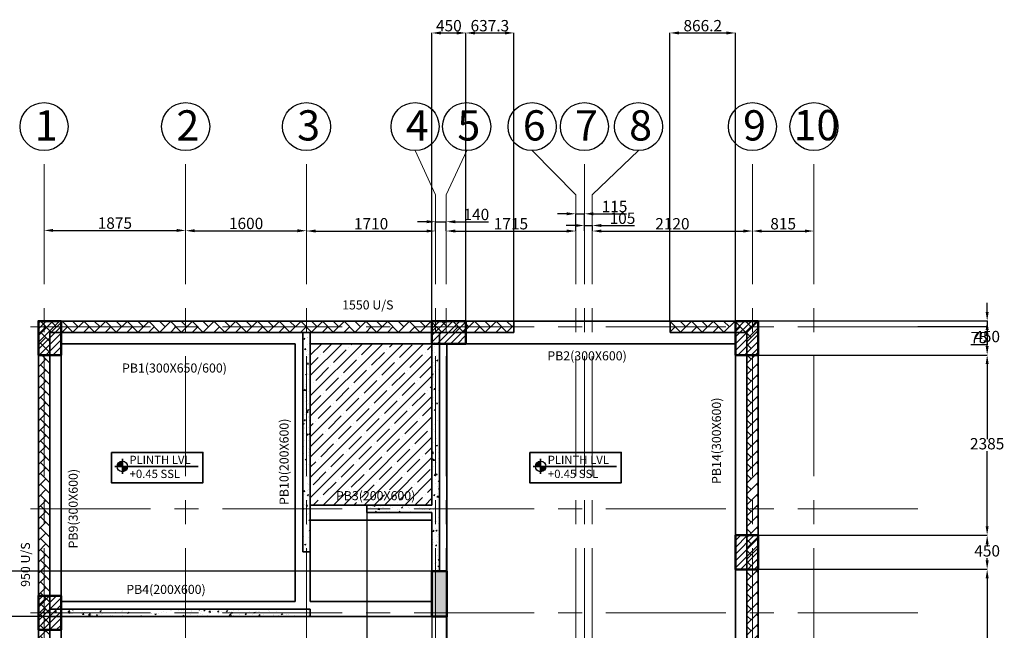
# Model space of a CAD drawing. Units: millimetres. Extents: x -174 to 32373, y 27344 to 53129.
# Tile 5 of 7: x 8204 to 21242, y 45053 to 53129. Entities that reach past the tile are written whole.
import ezdxf

# ---------------------------------------------------------------- set-up
doc = ezdxf.new("R2010")
doc.units = ezdxf.units.MM
doc.header["$LTSCALE"] = 50
doc.linetypes.add('CENTER', pattern=[50.8, 31.75, -6.35, 6.35, -6.35])
for name, color, linetype, lineweight in [('S-ANNO-DIMS', 2, 'Continuous', 18), ('S-ANNO-SYMB', 4, 'Continuous', 25), ('S-ANNO-TEXT', 3, 'Continuous', 18), ('S-BEAM', 7, 'Continuous', 35), ('S-COLS', 1, 'Continuous', 50), ('S-GRID', 8, 'CENTER', 18), ('S-GRID-IDEN', 7, 'Continuous', 25), ('S-PATT', 8, 'Continuous', 13)]:
    doc.layers.add(name, color=color, linetype=linetype, lineweight=lineweight)
doc.styles.get("Standard").update_dxf_attribs({"font": 'arial.ttf'})
doc.dimstyles.new('ISO-25', dxfattribs={"dimtxt": 150, "dimasz": 120, "dimexe": 1.25, "dimexo": 0.625, "dimtad": 1, "dimtih": 1, "dimtoh": 1, "dimdec": 0, "dimtxsty": 'Standard', "dimcen": 2.5, "dimadec": 0, "dimazin": 0, "dimtfac": 1, "dimtdec": 0, "dimtmove": 0, "dimatfit": 3, "dimfxl": 1, "dimarcsym": 0})

# ---------------------------------------------------------------- blocks, each defined once
blk = doc.blocks.new('*D1')
at = {"layer": 'Defpoints', "color": 0, "transparency": 16777216}
for p in [(8527, 50342), (10402, 50342), (10402, 50342)]:
    blk.add_point(p, dxfattribs=at)
at = {"layer": 'S-ANNO-DIMS', "color": 0, "lineweight": -2, "transparency": 16777216}
for p, q in [((8527, 50342), (8527, 50343)), ((8647, 50342), (10282, 50342)), ((10402, 50342), (10402, 50343))]:
    blk.add_line(p, q, dxfattribs=at)
at = {"layer": 'S-ANNO-DIMS', "color": 0, "transparency": 16777216}
for points in [[(8647, 50362), (8647, 50322), (8527, 50342)], [(10282, 50362), (10282, 50322), (10402, 50342)]]:
    blk.add_solid(points, dxfattribs=at)
at = {"layer": 'S-ANNO-DIMS', "color": 0, "transparency": 16777216, "insert": (9464, 50419), "char_height": 150, "attachment_point": 5}
blk.add_mtext('1875', dxfattribs=at)
blk = doc.blocks.new('*D2')
at = {"layer": 'Defpoints', "color": 0, "transparency": 16777216}
for p in [(10402, 50338), (12002, 50338), (12002, 50338)]:
    blk.add_point(p, dxfattribs=at)
at = {"layer": 'S-ANNO-DIMS', "color": 0, "lineweight": -2, "transparency": 16777216}
for p, q in [((10402, 50339), (10402, 50339)), ((10522, 50338), (11882, 50338)), ((12002, 50339), (12002, 50339))]:
    blk.add_line(p, q, dxfattribs=at)
at = {"layer": 'S-ANNO-DIMS', "color": 0, "transparency": 16777216}
for points in [[(10522, 50358), (10522, 50318), (10402, 50338)], [(11882, 50358), (11882, 50318), (12002, 50338)]]:
    blk.add_solid(points, dxfattribs=at)
at = {"layer": 'S-ANNO-DIMS', "color": 0, "transparency": 16777216, "insert": (11202, 50415), "char_height": 150, "attachment_point": 5}
blk.add_mtext('1600', dxfattribs=at)
blk = doc.blocks.new('*D3')
at = {"layer": 'Defpoints', "color": 0, "transparency": 16777216}
for p in [(12002, 50339), (13712, 50334), (13712, 50334)]:
    blk.add_point(p, dxfattribs=at)
at = {"layer": 'S-ANNO-DIMS', "color": 0, "lineweight": -2, "transparency": 16777216}
for p, q in [((12002, 50339), (12002, 50333)), ((12122, 50334), (13592, 50334)), ((13712, 50335), (13712, 50336))]:
    blk.add_line(p, q, dxfattribs=at)
at = {"layer": 'S-ANNO-DIMS', "color": 0, "transparency": 16777216}
for points in [[(12122, 50354), (12122, 50314), (12002, 50334)], [(13592, 50354), (13592, 50314), (13712, 50334)]]:
    blk.add_solid(points, dxfattribs=at)
at = {"layer": 'S-ANNO-DIMS', "color": 0, "transparency": 16777216, "insert": (12857, 50411), "char_height": 150, "attachment_point": 5}
blk.add_mtext('1710', dxfattribs=at)
blk = doc.blocks.new('*D4')
at = {"layer": 'Defpoints', "color": 0, "transparency": 16777216}
for p in [(13712, 50334), (13852, 50457), (13852, 50334)]:
    blk.add_point(p, dxfattribs=at)
at = {"layer": 'S-ANNO-DIMS', "color": 0, "lineweight": -2, "transparency": 16777216}
for p, q in [((13592, 50457), (13472, 50457)), ((13712, 50335), (13712, 50458)), ((13712, 50457), (13852, 50457)), ((13852, 50335), (13852, 50458)), ((13972, 50457), (14410, 50457))]:
    blk.add_line(p, q, dxfattribs=at)
at = {"layer": 'S-ANNO-DIMS', "color": 0, "transparency": 16777216}
for points in [[(13592, 50477), (13592, 50437), (13712, 50457)], [(13972, 50477), (13972, 50437), (13852, 50457)]]:
    blk.add_solid(points, dxfattribs=at)
at = {"layer": 'S-ANNO-DIMS', "color": 0, "transparency": 16777216, "insert": (14251, 50534), "char_height": 150, "attachment_point": 5}
blk.add_mtext('140', dxfattribs=at)
blk = doc.blocks.new('*D5')
at = {"layer": 'Defpoints', "color": 0, "transparency": 16777216}
for p in [(13852, 50334), (15567, 50334), (15567, 50334)]:
    blk.add_point(p, dxfattribs=at)
at = {"layer": 'S-ANNO-DIMS', "color": 0, "lineweight": -2, "transparency": 16777216}
for p, q in [((13852, 50335), (13852, 50336)), ((13972, 50334), (15447, 50334)), ((15567, 50335), (15567, 50336))]:
    blk.add_line(p, q, dxfattribs=at)
at = {"layer": 'S-ANNO-DIMS', "color": 0, "transparency": 16777216}
for points in [[(13972, 50354), (13972, 50314), (13852, 50334)], [(15447, 50354), (15447, 50314), (15567, 50334)]]:
    blk.add_solid(points, dxfattribs=at)
at = {"layer": 'S-ANNO-DIMS', "color": 0, "transparency": 16777216, "insert": (14709, 50411), "char_height": 150, "attachment_point": 5}
blk.add_mtext('1715', dxfattribs=at)
blk = doc.blocks.new('*D6')
at = {"layer": 'Defpoints', "color": 0, "transparency": 16777216}
for p in [(15682, 50562), (15567, 50334), (15682, 50334)]:
    blk.add_point(p, dxfattribs=at)
at = {"layer": 'S-ANNO-DIMS', "color": 0, "lineweight": -2, "transparency": 16777216}
for p, q in [((15447, 50562), (15327, 50562)), ((15567, 50335), (15567, 50563)), ((15567, 50562), (15682, 50562)), ((15682, 50335), (15682, 50563)), ((15802, 50562), (16241, 50562))]:
    blk.add_line(p, q, dxfattribs=at)
at = {"layer": 'S-ANNO-DIMS', "color": 0, "transparency": 16777216}
for points in [[(15447, 50582), (15447, 50542), (15567, 50562)], [(15802, 50582), (15802, 50542), (15682, 50562)]]:
    blk.add_solid(points, dxfattribs=at)
at = {"layer": 'S-ANNO-DIMS', "color": 0, "transparency": 16777216, "insert": (16081, 50639), "char_height": 150, "attachment_point": 5}
blk.add_mtext('115', dxfattribs=at)
blk = doc.blocks.new('*D7')
at = {"layer": 'Defpoints', "color": 0, "transparency": 16777216}
for p in [(15682, 50334), (15787, 50407), (15787, 50334)]:
    blk.add_point(p, dxfattribs=at)
at = {"layer": 'S-ANNO-DIMS', "color": 0, "lineweight": -2, "transparency": 16777216}
for p, q in [((15562, 50407), (15442, 50407)), ((15682, 50335), (15682, 50408)), ((15682, 50407), (15787, 50407)), ((15787, 50335), (15787, 50408)), ((15907, 50407), (16346, 50407))]:
    blk.add_line(p, q, dxfattribs=at)
at = {"layer": 'S-ANNO-DIMS', "color": 0, "transparency": 16777216}
for points in [[(15562, 50427), (15562, 50387), (15682, 50407)], [(15907, 50427), (15907, 50387), (15787, 50407)]]:
    blk.add_solid(points, dxfattribs=at)
at = {"layer": 'S-ANNO-DIMS', "color": 0, "transparency": 16777216, "insert": (16186, 50484), "char_height": 150, "attachment_point": 5}
blk.add_mtext('105', dxfattribs=at)
blk = doc.blocks.new('*D8')
at = {"layer": 'Defpoints', "color": 0, "transparency": 16777216}
for p in [(15787, 50334), (17907, 50334), (17907, 50334)]:
    blk.add_point(p, dxfattribs=at)
at = {"layer": 'S-ANNO-DIMS', "color": 0, "lineweight": -2, "transparency": 16777216}
for p, q in [((15787, 50335), (15787, 50336)), ((15907, 50334), (17787, 50334)), ((17907, 50335), (17907, 50336))]:
    blk.add_line(p, q, dxfattribs=at)
at = {"layer": 'S-ANNO-DIMS', "color": 0, "transparency": 16777216}
for points in [[(15907, 50354), (15907, 50314), (15787, 50334)], [(17787, 50354), (17787, 50314), (17907, 50334)]]:
    blk.add_solid(points, dxfattribs=at)
at = {"layer": 'S-ANNO-DIMS', "color": 0, "transparency": 16777216, "insert": (16847, 50411), "char_height": 150, "attachment_point": 5}
blk.add_mtext('2120', dxfattribs=at)
blk = doc.blocks.new('*D9')
at = {"layer": 'Defpoints', "color": 0, "transparency": 16777216}
for p in [(17907, 50334), (18722, 50334), (18722, 50334)]:
    blk.add_point(p, dxfattribs=at)
at = {"layer": 'S-ANNO-DIMS', "color": 0, "lineweight": -2, "transparency": 16777216}
for p, q in [((17907, 50335), (17907, 50336)), ((18027, 50334), (18602, 50334)), ((18722, 50335), (18722, 50336))]:
    blk.add_line(p, q, dxfattribs=at)
at = {"layer": 'S-ANNO-DIMS', "color": 0, "transparency": 16777216}
for points in [[(18027, 50354), (18027, 50314), (17907, 50334)], [(18602, 50354), (18602, 50314), (18722, 50334)]]:
    blk.add_solid(points, dxfattribs=at)
at = {"layer": 'S-ANNO-DIMS', "color": 0, "transparency": 16777216, "insert": (18314, 50411), "char_height": 150, "attachment_point": 5}
blk.add_mtext('815', dxfattribs=at)
blk = doc.blocks.new('*D39')
at = {"layer": 'Defpoints', "color": 0, "transparency": 16777216}
for p in [(17982, 49144), (20095, 49069), (21015, 49069)]:
    blk.add_point(p, dxfattribs=at)
at = {"layer": 'S-ANNO-DIMS', "color": 0, "lineweight": -2, "transparency": 16777216}
for p, q in [((21015, 49264), (21015, 49384)), ((17982, 49144), (21016, 49144)), ((20096, 49069), (21016, 49069)), ((21015, 49144), (21015, 49069)), ((21015, 48949), (21015, 48829)), ((21015, 48829), (20800, 48829))]:
    blk.add_line(p, q, dxfattribs=at)
at = {"layer": 'S-ANNO-DIMS', "color": 0, "transparency": 16777216}
for points in [[(20995, 49264), (21035, 49264), (21015, 49144)], [(20995, 48949), (21035, 48949), (21015, 49069)]]:
    blk.add_solid(points, dxfattribs=at)
at = {"layer": 'S-ANNO-DIMS', "color": 0, "transparency": 16777216, "insert": (20907, 48906), "char_height": 150, "attachment_point": 5}
blk.add_mtext('75', dxfattribs=at)
blk = doc.blocks.new('*D40')
at = {"layer": 'Defpoints', "color": 0, "transparency": 16777216}
for p in [(17982, 49144), (17982, 48694), (21015, 48694)]:
    blk.add_point(p, dxfattribs=at)
at = {"layer": 'S-ANNO-DIMS', "color": 0, "lineweight": -2, "transparency": 16777216}
for p, q in [((17982, 49144), (21016, 49144)), ((21015, 49024), (21015, 48996)), ((21015, 48814), (21015, 48842)), ((17982, 48694), (21016, 48694))]:
    blk.add_line(p, q, dxfattribs=at)
at = {"layer": 'S-ANNO-DIMS', "color": 0, "transparency": 16777216}
for points in [[(20995, 49024), (21035, 49024), (21015, 49144)], [(20995, 48814), (21035, 48814), (21015, 48694)]]:
    blk.add_solid(points, dxfattribs=at)
at = {"layer": 'S-ANNO-DIMS', "color": 0, "transparency": 16777216, "insert": (21015, 48919), "char_height": 150, "attachment_point": 5}
blk.add_mtext('450', dxfattribs=at)
blk = doc.blocks.new('*D42')
at = {"layer": 'Defpoints', "color": 0, "transparency": 16777216}
for p in [(14112, 52954), (13662, 49144), (14112, 49144)]:
    blk.add_point(p, dxfattribs=at)
at = {"layer": 'S-ANNO-DIMS', "color": 0, "lineweight": -2, "transparency": 16777216}
for p, q in [((13662, 49144), (13662, 52955)), ((13782, 52954), (13992, 52954)), ((14112, 49144), (14112, 52955))]:
    blk.add_line(p, q, dxfattribs=at)
at = {"layer": 'S-ANNO-DIMS', "color": 0, "transparency": 16777216}
for points in [[(13782, 52974), (13782, 52934), (13662, 52954)], [(13992, 52974), (13992, 52934), (14112, 52954)]]:
    blk.add_solid(points, dxfattribs=at)
at = {"layer": 'S-ANNO-DIMS', "color": 0, "transparency": 16777216, "insert": (13887, 53031), "char_height": 150, "attachment_point": 5}
blk.add_mtext('450', dxfattribs=at)
blk = doc.blocks.new('*D44')
at = {"layer": 'Defpoints', "color": 0, "transparency": 16777216}
for p in [(13662, 45234), (13862, 45234), (13862, 34336)]:
    blk.add_point(p, dxfattribs=at)
at = {"layer": 'S-ANNO-DIMS', "color": 0, "lineweight": -2, "transparency": 16777216}
for p, q in [((13662, 45233), (13662, 34335)), ((13862, 45233), (13862, 34335)), ((13542, 34336), (13422, 34336)), ((13662, 34336), (13862, 34336)), ((13982, 34336), (14436, 34336))]:
    blk.add_line(p, q, dxfattribs=at)
at = {"layer": 'S-ANNO-DIMS', "color": 0, "transparency": 16777216}
for points in [[(13542, 34356), (13542, 34316), (13662, 34336)], [(13982, 34356), (13982, 34316), (13862, 34336)]]:
    blk.add_solid(points, dxfattribs=at)
at = {"layer": 'S-ANNO-DIMS', "color": 0, "transparency": 16777216, "insert": (14269, 34413), "char_height": 150, "attachment_point": 5}
blk.add_mtext('200', dxfattribs=at)
blk = doc.blocks.new('*D45')
at = {"layer": 'Defpoints', "color": 0, "transparency": 16777216}
for p in [(1935, 45834), (13662, 45834), (13662, 45234)]:
    blk.add_point(p, dxfattribs=at)
at = {"layer": 'S-ANNO-DIMS', "color": 0, "lineweight": -2, "transparency": 16777216}
for p, q in [((13661, 45834), (1934, 45834)), ((1935, 45714), (1935, 45611)), ((1935, 45354), (1935, 45457)), ((13661, 45234), (1934, 45234))]:
    blk.add_line(p, q, dxfattribs=at)
at = {"layer": 'S-ANNO-DIMS', "color": 0, "transparency": 16777216}
for points in [[(1915, 45714), (1955, 45714), (1935, 45834)], [(1915, 45354), (1955, 45354), (1935, 45234)]]:
    blk.add_solid(points, dxfattribs=at)
at = {"layer": 'S-ANNO-DIMS', "color": 0, "transparency": 16777216, "insert": (1935, 45534), "char_height": 150, "attachment_point": 5}
blk.add_mtext('600', dxfattribs=at)
blk = doc.blocks.new('*D50')
at = {"layer": 'Defpoints', "color": 0, "transparency": 16777216}
for p in [(17982, 48694), (17982, 46309), (21015, 46309)]:
    blk.add_point(p, dxfattribs=at)
at = {"layer": 'S-ANNO-DIMS', "color": 0, "lineweight": -2, "transparency": 16777216}
for p, q in [((17982, 48694), (21016, 48694)), ((21015, 48574), (21015, 47579)), ((21015, 46429), (21015, 47424)), ((17982, 46309), (21016, 46309))]:
    blk.add_line(p, q, dxfattribs=at)
at = {"layer": 'S-ANNO-DIMS', "color": 0, "transparency": 16777216}
for points in [[(20995, 48574), (21035, 48574), (21015, 48694)], [(20995, 46429), (21035, 46429), (21015, 46309)]]:
    blk.add_solid(points, dxfattribs=at)
at = {"layer": 'S-ANNO-DIMS', "color": 0, "transparency": 16777216, "insert": (21015, 47501), "char_height": 150, "attachment_point": 5}
blk.add_mtext('2385', dxfattribs=at)
blk = doc.blocks.new('*D51')
at = {"layer": 'Defpoints', "color": 0, "transparency": 16777216}
for p in [(17982, 46309), (17982, 45859), (21015, 45859)]:
    blk.add_point(p, dxfattribs=at)
at = {"layer": 'S-ANNO-DIMS', "color": 0, "lineweight": -2, "transparency": 16777216}
for p, q in [((17982, 46309), (21016, 46309)), ((21015, 46189), (21015, 46161)), ((21015, 45979), (21015, 46007)), ((17982, 45859), (21016, 45859))]:
    blk.add_line(p, q, dxfattribs=at)
at = {"layer": 'S-ANNO-DIMS', "color": 0, "transparency": 16777216}
for points in [[(20995, 46189), (21035, 46189), (21015, 46309)], [(20995, 45979), (21035, 45979), (21015, 45859)]]:
    blk.add_solid(points, dxfattribs=at)
at = {"layer": 'S-ANNO-DIMS', "color": 0, "transparency": 16777216, "insert": (21015, 46084), "char_height": 150, "attachment_point": 5}
blk.add_mtext('450', dxfattribs=at)
blk = doc.blocks.new('*D52')
at = {"layer": 'Defpoints', "color": 0, "transparency": 16777216}
for p in [(17982, 45859), (17982, 43474), (21015, 43474)]:
    blk.add_point(p, dxfattribs=at)
at = {"layer": 'S-ANNO-DIMS', "color": 0, "lineweight": -2, "transparency": 16777216}
for p, q in [((17982, 45859), (21016, 45859)), ((21015, 45739), (21015, 44744)), ((21015, 43594), (21015, 44589)), ((17982, 43474), (21016, 43474))]:
    blk.add_line(p, q, dxfattribs=at)
at = {"layer": 'S-ANNO-DIMS', "color": 0, "transparency": 16777216}
for points in [[(20995, 45739), (21035, 45739), (21015, 45859)], [(20995, 43594), (21035, 43594), (21015, 43474)]]:
    blk.add_solid(points, dxfattribs=at)
at = {"layer": 'S-ANNO-DIMS', "color": 0, "transparency": 16777216, "insert": (21015, 44666), "char_height": 150, "attachment_point": 5}
blk.add_mtext('2385', dxfattribs=at)
blk = doc.blocks.new('*D54')
at = {"layer": 'Defpoints', "color": 0, "transparency": 16777216}
for p in [(14749, 52954), (14112, 49144), (14749, 49144)]:
    blk.add_point(p, dxfattribs=at)
at = {"layer": 'S-ANNO-DIMS', "color": 0, "lineweight": -2, "transparency": 16777216}
for p, q in [((14112, 49144), (14112, 52955)), ((14232, 52954), (14629, 52954)), ((14749, 49144), (14749, 52955))]:
    blk.add_line(p, q, dxfattribs=at)
at = {"layer": 'S-ANNO-DIMS', "color": 0, "transparency": 16777216}
for points in [[(14232, 52974), (14232, 52934), (14112, 52954)], [(14629, 52974), (14629, 52934), (14749, 52954)]]:
    blk.add_solid(points, dxfattribs=at)
at = {"layer": 'S-ANNO-DIMS', "color": 0, "transparency": 16777216, "insert": (14430, 53031), "char_height": 150, "attachment_point": 5}
blk.add_mtext('637.3', dxfattribs=at)
blk = doc.blocks.new('*D55')
at = {"layer": 'Defpoints', "color": 0, "transparency": 16777216}
for p in [(17682, 52954), (16815, 49144), (17682, 49144)]:
    blk.add_point(p, dxfattribs=at)
at = {"layer": 'S-ANNO-DIMS', "color": 0, "lineweight": -2, "transparency": 16777216}
for p, q in [((16815, 49144), (16815, 52955)), ((16935, 52954), (17562, 52954)), ((17682, 49144), (17682, 52955))]:
    blk.add_line(p, q, dxfattribs=at)
at = {"layer": 'S-ANNO-DIMS', "color": 0, "transparency": 16777216}
for points in [[(16935, 52974), (16935, 52934), (16815, 52954)], [(17562, 52974), (17562, 52934), (17682, 52954)]]:
    blk.add_solid(points, dxfattribs=at)
at = {"layer": 'S-ANNO-DIMS', "color": 0, "transparency": 16777216, "insert": (17249, 53031), "char_height": 150, "attachment_point": 5}
blk.add_mtext('866.2', dxfattribs=at)
blk = doc.blocks.new('*D59')
at = {"layer": 'Defpoints', "color": 0, "transparency": 16777216}
for p in [(12800, 46609), (13662, 46609), (13662, 34336)]:
    blk.add_point(p, dxfattribs=at)
at = {"layer": 'S-ANNO-DIMS', "color": 0, "lineweight": -2, "transparency": 16777216}
for p, q in [((12800, 46608), (12800, 34335)), ((13662, 46608), (13662, 34335)), ((12920, 34336), (13542, 34336))]:
    blk.add_line(p, q, dxfattribs=at)
at = {"layer": 'S-ANNO-DIMS', "color": 0, "transparency": 16777216}
for points in [[(12920, 34356), (12920, 34316), (12800, 34336)], [(13542, 34356), (13542, 34316), (13662, 34336)]]:
    blk.add_solid(points, dxfattribs=at)
at = {"layer": 'S-ANNO-DIMS', "color": 0, "transparency": 16777216, "insert": (13231, 34413), "char_height": 150, "attachment_point": 5}
blk.add_mtext('862', dxfattribs=at)

msp = doc.modelspace()

# ---------------------------------------------------------------- hatches: boundary and pattern name
at = {"layer": 'S-PATT'}
h = msp.add_hatch(dxfattribs=at)
h.set_pattern_fill('ANSI31', color=256, scale=20)
h.paths.add_polyline_path([(8751.66, 49143.76), (8451.66, 49143.76), (8451.66, 48693.76), (8751.66, 48693.76)])
h = msp.add_hatch(dxfattribs=at)
h.set_pattern_fill('AR-HBONE', color=256)
h.paths.add_polyline_path([(8601.66, 48993.76), (14749, 48993.76), (14749, 49143.76), (8451.66, 49143.76), (8451.66, 41103.32), (8601.66, 41103.32)])
h = msp.add_hatch(dxfattribs=at)
h.set_pattern_fill('ANSI31', color=256, scale=20)
h.paths.add_polyline_path([(14111.66, 49143.76), (13661.66, 49143.76), (13661.66, 48843.76), (14111.66, 48843.76)])
h = msp.add_hatch(dxfattribs=at)
h.set_pattern_fill('AR-HBONE', color=256)
h.paths.add_polyline_path([(17981.66, 49143.76), (16815.46, 49143.76), (16815.46, 48993.76), (17831.66, 48993.76), (17831.66, 43173.76), (17681.66, 43173.76), (17681.66, 43023.76), (17981.66, 43023.76)])
h = msp.add_hatch(dxfattribs=at)
h.set_pattern_fill('ANSI31', color=256, scale=20)
h.paths.add_polyline_path([(17981.66, 49143.76), (17681.66, 49143.76), (17681.66, 48693.76), (17981.66, 48693.76)])
h = msp.add_hatch(dxfattribs=at)
h.set_pattern_fill('AR-CONC', color=256)
h.paths.add_polyline_path([(12051.66, 46708.76), (12051.66, 48993.76), (11951.66, 48993.76), (11951.66, 46091.85), (12051.66, 46091.85), (12051.66, 46508.76)])
h = msp.add_hatch(dxfattribs=at)
h.set_pattern_fill('AR-CONC', color=256)
h.paths.add_polyline_path([(13761.66, 48993.76), (13661.66, 48993.76), (13661.66, 46708.76), (12799.66, 46708.76), (12799.66, 46608.76), (13661.66, 46608.76), (13661.66, 46508.76), (13661.66, 45833.76), (13761.66, 45833.76)])
h = msp.add_hatch(dxfattribs=at)
h.set_pattern_fill('ANSI35', color=256, scale=30)
h.paths.add_polyline_path([(13661.66, 48843.76), (12051.66, 48843.76), (12051.66, 46708.76), (13661.66, 46708.76)])
h.paths.add_polyline_path([(12348.44, 46705.85), (13508.17, 46705.85), (13508.17, 46953.14), (12348.44, 46953.14)], flags=9)
h = msp.add_hatch(color=256, dxfattribs=at)
h.dxf.hatch_style = 1
h.paths.add_polyline_path([(9563.15, 47288.57, 0.41421356), (9494.18, 47219.6), (9563.15, 47219.6)])
h.paths.add_polyline_path([(9563.15, 47219.6), (9563.15, 47150.63, 0.41421356), (9632.13, 47219.6)])
h = msp.add_hatch(color=256, dxfattribs=at)
h.dxf.hatch_style = 1
h.paths.add_polyline_path([(15102.63, 47288.57, 0.41421356), (15033.65, 47219.6), (15102.63, 47219.6)])
h.paths.add_polyline_path([(15102.63, 47219.6), (15102.63, 47150.63, 0.41421356), (15171.6, 47219.6)])
h = msp.add_hatch(dxfattribs=at)
h.set_pattern_fill('ANSI31', color=256, scale=20)
h.paths.add_polyline_path([(17981.66, 46308.76), (17681.66, 46308.76), (17681.66, 45858.76), (17981.66, 45858.76)])
h = msp.add_hatch(color=256, dxfattribs=at)
h.dxf.hatch_style = 1
h.paths.add_polyline_path([(13861.66, 45833.76), (13661.66, 45833.76), (13661.66, 45233.76), (13861.66, 45233.76)])
h = msp.add_hatch(dxfattribs=at)
h.set_pattern_fill('ANSI31', color=256, scale=20)
h.paths.add_polyline_path([(8751.66, 45508.76), (8451.66, 45508.76), (8451.66, 45058.76), (8751.66, 45058.76)])
h = msp.add_hatch(dxfattribs=at)
h.set_pattern_fill('AR-CONC', color=256)
h.paths.add_polyline_path([(12051.66, 45333.76), (8601.66, 45333.76), (8601.66, 45233.76), (12051.66, 45233.76)])

# ---------------------------------------------------------------- linework, layer by layer
at = {"layer": 'S-ANNO-SYMB'}
for centre in [(9563.15, 47219.6), (15102.63, 47219.6)]:
    msp.add_circle(centre, 68.97, dxfattribs=at)
at = {"layer": 'S-BEAM'}
for p, q in [((8451.66, 38443.76), (8451.66, 49143.76)), ((17981.66, 49143.76), (8451.66, 49143.76)), ((14749, 48993.76), (14749, 49143.76)), ((16815.46, 48993.76), (16815.46, 49143.76)), ((17981.66, 43023.76), (17981.66, 49143.76)), ((14749, 48993.76), (8601.66, 48993.76)), ((11951.66, 46091.85), (11951.66, 48993.76)), ((12051.66, 46708.76), (12051.66, 48993.76)), ((17831.66, 48993.76), (16815.46, 48993.76)), ((17831.66, 43173.76), (17831.66, 48993.76)), ((11851.66, 48843.76), (8751.66, 48843.76)), ((8751.66, 45433.76), (8751.66, 48843.76)), ((11851.66, 45433.76), (11851.66, 48843.76)), ((13661.66, 48843.76), (12051.66, 48843.76)), ((13861.66, 45233.76), (13861.66, 48843.76)), ((17681.66, 48843.76), (13861.66, 48843.76)), ((17681.66, 43323.76), (17681.66, 48843.76)), ((9464.18, 47219.6), (10566.86, 47219.6)), ((9563.15, 47318.57), (9563.15, 47120.63)), ((15003.65, 47219.6), (16106.33, 47219.6)), ((15102.63, 47318.57), (15102.63, 47120.63)), ((13661.66, 46708.76), (12051.66, 46708.76)), ((12051.66, 46508.76), (12051.66, 46708.76)), ((12799.66, 46708.76), (12799.66, 46608.76)), ((13661.66, 46608.76), (12799.66, 46608.76)), ((13661.66, 46508.76), (13661.66, 46608.76)), ((13661.66, 46508.76), (12051.66, 46508.76)), ((12051.66, 45433.76), (12051.66, 46508.76)), ((11951.66, 46091.85), (12051.66, 46091.85)), ((13761.66, 45833.76), (13661.66, 45833.76)), ((11851.66, 45433.76), (8751.66, 45433.76)), ((13661.66, 45433.76), (12051.66, 45433.76)), ((12051.66, 45333.76), (8601.66, 45333.76)), ((12051.66, 45233.76), (12051.66, 45333.76)), ((13861.66, 45233.76), (8601.66, 45233.76)), ((8751.66, 38743.76), (8751.66, 45233.76))]:
    msp.add_line(p, q, dxfattribs=at)
for points in [[(8601.66, 48993.76), (8601.66, 41103.32)], [(13661.66, 46708.76), (13661.66, 48993.76)], [(13761.66, 45833.76), (13761.66, 48993.76)], [(13661.66, 45433.76), (13661.66, 46508.76)]]:
    msp.add_lwpolyline(points, dxfattribs=at)
for points in [[(9418.46, 47405.35), (10630.8, 47405.35), (10630.8, 47004.4), (9418.46, 47004.4)], [(14957.93, 47405.35), (16170.27, 47405.35), (16170.27, 47004.4), (14957.93, 47004.4)]]:
    msp.add_lwpolyline(points, close=True, dxfattribs=at)
at = {"layer": 'S-COLS'}
for points in [[(8451.66, 48693.76), (8751.66, 48693.76), (8751.66, 49143.76), (8451.66, 49143.76)], [(13661.66, 49143.76), (13661.66, 48843.76), (14111.66, 48843.76), (14111.66, 49143.76)], [(17681.66, 48693.76), (17981.66, 48693.76), (17981.66, 49143.76), (17681.66, 49143.76)], [(17681.66, 45858.76), (17981.66, 45858.76), (17981.66, 46308.76), (17681.66, 46308.76)], [(13661.66, 45233.76), (13861.66, 45233.76), (13861.66, 45833.76), (13661.66, 45833.76)], [(8451.66, 45058.76), (8751.66, 45058.76), (8751.66, 45508.76), (8451.66, 45508.76)]]:
    msp.add_lwpolyline(points, close=True, dxfattribs=at)
at = {"layer": 'S-GRID'}
for p, q in [((8526.66, 36931.64), (8526.66, 51397.21)), ((10401.66, 36931.64), (10401.66, 51397.21)), ((12001.66, 36931.64), (12001.66, 51397.21)), ((15681.66, 36931.64), (15681.66, 51397.21)), ((17906.66, 36931.64), (17906.66, 51397.21)), ((18721.66, 36931.64), (18721.66, 51397.21)), ((20095.15, 49068.76), (3491.75, 49068.76)), ((20095.15, 46658.76), (3491.75, 46658.76)), ((20095.15, 45283.76), (3491.75, 45283.76))]:
    msp.add_line(p, q, dxfattribs=at)
for points in [[(13711.66, 36931.64), (13711.66, 50814.23), (13439.61, 51397.21)], [(13851.66, 36931.64), (13851.66, 50814.23), (14122.87, 51397.21)], [(15566.66, 36931.64), (15566.66, 50814.23), (14989.62, 51397.21)], [(15786.66, 36931.64), (15786.66, 50814.23), (16397.9, 51397.21)]]:
    msp.add_lwpolyline(points, dxfattribs=at)
at = {"layer": 'S-GRID-IDEN'}
for centre in [(8526.66, 51715.39), (10401.66, 51715.39), (12001.66, 51715.39), (13439.61, 51715.39), (14122.87, 51715.39), (14989.62, 51715.39), (15681.66, 51715.39), (16397.9, 51715.39), (17906.66, 51715.39), (18721.66, 51715.39)]:
    msp.add_circle(centre, 318.18, dxfattribs=at)

# ---------------------------------------------------------------- texts
at = {"layer": 'S-ANNO-TEXT'}
for s, p in [('PLINTH LVL', (9656.07, 47251.71)), ('PLINTH LVL', (15195.54, 47251.71)), ('+0.45 SSL', (9659.37, 47066.5)), ('+0.45 SSL', (15198.84, 47066.5))]:
    msp.add_text(s, height=110, dxfattribs=at).set_placement(p)
at = {"layer": 'S-ANNO-TEXT', "char_height": 120, "attachment_point": 1}
for s, insert in [('1550 U/S', (12473.64, 49416.63)), ('PB2(300X600)', (15191.03, 48743.18)), ('PB1(300X650/600)', (9559.26, 48581.75)), ('PB3(200X600)', (12391.37, 46893.43)), ('PB4(200X600)', (9615.39, 45653.73))]:
    msp.add_mtext_dynamic_manual_height_columns(s, width=1913.0414, gutter_width=12.5, heights=[0], dxfattribs=dict(at, insert=insert))
at = {"layer": 'S-ANNO-TEXT', "char_height": 120, "attachment_point": 1, "rotation": 90}
for s, insert in [('PB14(300X600)', (17370.22, 46988.57)), ('PB10(200X600)', (11644.64, 46710.45)), ('PB9(300X600)', (8852.21, 46135.49)), ('950 U/S', (8220.17, 45627.06))]:
    msp.add_mtext_dynamic_manual_height_columns(s, width=1913.0414, gutter_width=12.5, heights=[0], dxfattribs=dict(at, insert=insert))
at = {"layer": 'S-GRID-IDEN', "char_height": 400, "attachment_point": 1}
for s, insert in [('1', (8403.45, 51931.46)), ('2', (10278.45, 51931.46)), ('3', (11878.45, 51931.46)), ('4', (13316.4, 51931.46)), ('5', (13999.66, 51931.46)), ('6', (14866.4, 51931.46)), ('7', (15558.45, 51931.46)), ('8', (16274.69, 51931.46)), ('9', (17783.45, 51931.46)), ('10', (18451.31, 51935.13))]:
    msp.add_mtext_dynamic_manual_height_columns(s, width=343.3972, gutter_width=12.5, heights=[0], dxfattribs=dict(at, insert=insert))

# ---------------------------------------------------------------- dimensions: what is measured, and where the dimension line sits
at = {"layer": 'S-ANNO-DIMS'}
for base, p1, p2, override, picture, middle in [((14111.66, 52953.58), (13661.66, 49143.76), (14111.66, 49143.76), {"dimdec": 0, "dimlfac": 1, "dimrnd": 0, "dimzin": 0, "dimdsep": 46, "dimlunit": 2}, '*D42', (13886.66, 53030.79)), ((14749, 52953.58), (14111.66, 49143.76), (14749, 49143.76), {"dimdec": 1, "dimlfac": 1, "dimrnd": 0, "dimzin": 0, "dimdsep": 46, "dimlunit": 2}, '*D54', (14430.33, 53030.84)), ((17681.66, 52953.58), (16815.46, 49143.76), (17681.66, 49143.76), {"dimdec": 1, "dimlfac": 1, "dimrnd": 0, "dimzin": 0, "dimdsep": 46, "dimlunit": 2}, '*D55', (17248.56, 53030.79)), ((15681.66, 50561.81), (15566.66, 50334.27), (15681.66, 50334.27), {"dimclrd": 0, "dimclre": 0, "dimclrt": 0}, '*D6', (16081.5, 50639.03)), ((13851.66, 50456.86), (13711.66, 50334.27), (13851.66, 50334.27), {"dimclrd": 0, "dimclre": 0, "dimclrt": 0}, '*D4', (14250.68, 50534.07)), ((10401.66, 50341.77), (8526.66, 50341.77), (10401.66, 50341.77), {"dimclrd": 0, "dimclre": 0, "dimclrt": 0}, '*D1', (9464.16, 50418.98)), ((12001.66, 50338.02), (10401.66, 50338.02), (12001.66, 50338.02), {"dimclrd": 0, "dimclre": 0, "dimclrt": 0}, '*D2', (11201.66, 50415.23)), ((13711.66, 50334.27), (12001.66, 50339.27), (13711.66, 50334.27), {"dimclrd": 0, "dimclre": 0, "dimclrt": 0}, '*D3', (12856.66, 50411.48)), ((15566.66, 50334.27), (13851.66, 50334.27), (15566.66, 50334.27), {"dimclrd": 0, "dimclre": 0, "dimclrt": 0}, '*D5', (14709.16, 50411.48)), ((15786.66, 50406.78), (15681.66, 50334.27), (15786.66, 50334.27), {"dimclrd": 0, "dimclre": 0, "dimclrt": 0}, '*D7', (16186.5, 50483.99)), ((17906.66, 50334.27), (15786.66, 50334.27), (17906.66, 50334.27), {"dimclrd": 0, "dimclre": 0, "dimclrt": 0}, '*D8', (16846.66, 50411.48)), ((18721.66, 50334.27), (17906.66, 50334.27), (18721.66, 50334.27), {"dimclrd": 0, "dimclre": 0, "dimclrt": 0}, '*D9', (18314.16, 50411.48)), ((13661.66, 34335.75), (12799.66, 46608.76), (13661.66, 46608.76), {"dimdec": 0, "dimlfac": 1, "dimrnd": 0, "dimzin": 0, "dimdsep": 46, "dimlunit": 2}, '*D59', (13230.66, 34412.96)), ((13861.66, 34335.75), (13661.66, 45233.76), (13861.66, 45233.76), {"dimdec": 0, "dimlfac": 1, "dimrnd": 0, "dimzin": 0, "dimdsep": 46, "dimlunit": 2}, '*D44', (14269.02, 34412.96))]:
    dim = msp.add_linear_dim(base=base, p1=p1, p2=p2, dimstyle='ISO-25', override=override, dxfattribs=at)
    dim.commit()
    dim.dimension.update_dxf_attribs({"geometry": picture, "text_midpoint": middle})
for base, p1, p2, picture, middle in [((21015.15, 49068.76), (17981.66, 49143.76), (20095.15, 49068.76), '*D39', (20907.14, 48905.66)), ((21015.15, 48693.76), (17981.66, 49143.76), (17981.66, 48693.76), '*D40', (21015.15, 48918.76)), ((21015.15, 46308.76), (17981.66, 48693.76), (17981.66, 46308.76), '*D50', (21015.15, 47501.26)), ((21015.15, 45858.76), (17981.66, 46308.76), (17981.66, 45858.76), '*D51', (21015.15, 46083.76)), ((1935.38, 45833.76), (13661.66, 45233.76), (13661.66, 45833.76), '*D45', (1935.38, 45533.76)), ((21015.15, 43473.76), (17981.66, 45858.76), (17981.66, 43473.76), '*D52', (21015.15, 44666.26))]:
    dim = msp.add_linear_dim(base=base, p1=p1, p2=p2, angle=90, dimstyle='ISO-25', override={"dimdec": 0, "dimlfac": 1, "dimrnd": 0, "dimzin": 0, "dimdsep": 46, "dimlunit": 2}, dxfattribs=at)
    dim.commit()
    dim.dimension.update_dxf_attribs({"geometry": picture, "text_midpoint": middle})

doc.saveas('drawing.dxf')
